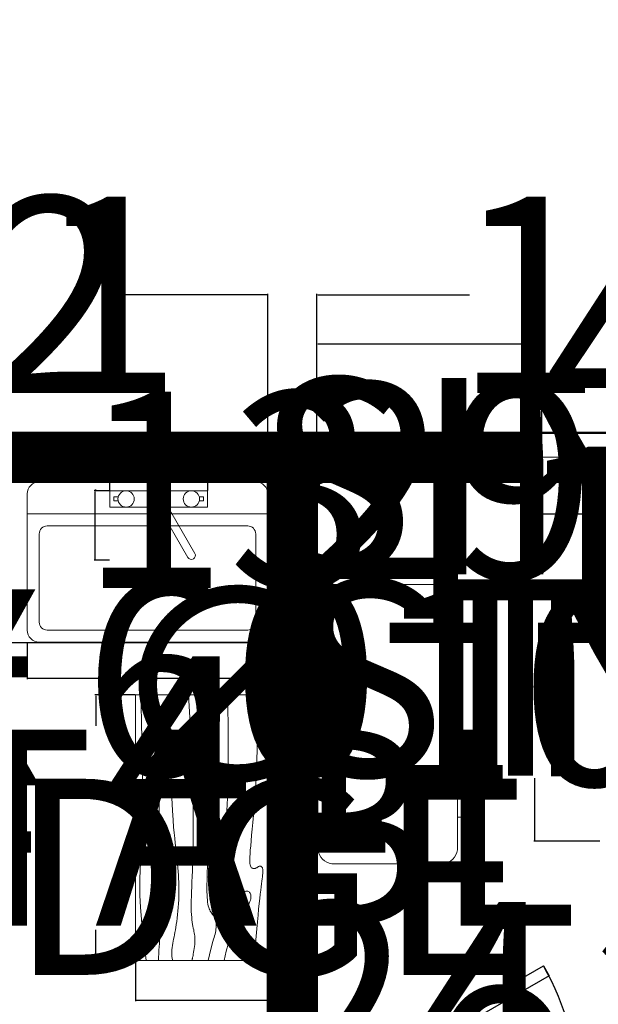
# Model space of a CAD drawing. Units: inches. Extents: x 1173 to 2157, y 515 to 1129.
# Tile 10 of 13: x 1475 to 1581, y 948 to 1129. Entities that reach past the tile are written whole.
import ezdxf

# ---------------------------------------------------------------- set-up
doc = ezdxf.new("R2010")
doc.units = ezdxf.units.IN
doc.header["$MEASUREMENT"] = 0
for name, color, linetype, lineweight in [('A-ANNO-DIMS', 2, 'Continuous', 18), ('A-DOOR', 3, 'Continuous', 25), ('A-FLOR-CASE', 32, 'Continuous', 25), ('A-FLOR-FIXT', 9, 'Continuous', 18), ('A-FURN', 8, 'Continuous', 18), ('A-GLAZ', 4, 'Continuous', 18), ('A-WALL', 7, 'Continuous', 50)]:
    doc.layers.add(name, color=color, linetype=linetype, lineweight=lineweight)
doc.layers.add('A-WALL-PATT', color=22, linetype='Continuous', lineweight=13, true_color=0xca4b0c)
doc.styles.get("Standard").update_dxf_attribs({"font": 'arial.ttf'})
doc.dimstyles.get("Standard").update_dxf_attribs({"dimtxt": 36, "dimasz": 0.18, "dimexe": 0.18, "dimexo": 0.0625, "dimgap": 0.09, "dimtad": 0, "dimtih": 1, "dimtoh": 1, "dimdec": 0, "dimrnd": 72, "dimzin": 0, "dimdsep": 46, "dimlunit": 3, "dimtxsty": 'Standard', "dimcen": 2, "dimadec": 0, "dimazin": 0, "dimtfac": 1, "dimtdec": 0, "dimtofl": 0, "dimtmove": 0, "dimatfit": 3, "dimfxl": 1, "dimtolj": 1, "dimtzin": 0, "dimarcsym": 0})

# ---------------------------------------------------------------- blocks, each defined once
blk = doc.blocks.new('*U3')
for p, q in [((0, 0), (0, -6)), ((40, 0), (40, -6))]:
    blk.add_line(p, q)
blk.add_lwpolyline([(0, 0), (34.64, 20), (35.52, 18.48), (0.88, -1.52)], close=True)
blk.add_arc((0, 0), 40, 0, 30)
blk = doc.blocks.new('Desk - 30 x 60 in.')
for p, q in [((-26.999995, 0), (26.999995, 0)), ((-29.999995, -27), (-29.999995, -3)), ((29.999995, -3), (29.999995, -27)), ((26.999995, -30), (-26.999995, -30)), ((-20.000005, -30), (-20.000005, -31)), ((-20.000005, -31), (-16.000005, -31)), ((-16.000005, -31), (-16.000005, -30)), ((15.999995, -31), (15.999995, -30)), ((19.999995, -31), (15.999995, -31)), ((19.999995, -30), (19.999995, -31))]:
    blk.add_line(p, q)
for centre, start, end in [((-26.499995, -3.5), 98.1301, 171.8699), ((26.499995, -3.5), 8.130102, 81.8699), ((-26.499995, -26.5), 188.1301, 261.8699), ((26.499995, -26.5), 278.1301, 351.8699)]:
    blk.add_arc(centre, 3.535534, start, end)
blk = doc.blocks.new('Table - Rectangular Woodgrain 60 x 30 in.')
for p, q in [((0, 0), (0, -30)), ((60, 0), (0, 0)), ((60, -30), (60, 0)), ((0, -30), (60, -30))]:
    blk.add_line(p, q)
for points in [[(0, -2.4), (4.8155, -2.418), (9.0302, -2.4688), (12.709, -2.5477), (15.9167, -2.65), (18.7181, -2.7711), (21.1781, -2.9063), (23.3616, -3.0508), (25.3333, -3.2), (27.1477, -3.3495), (28.8172, -3.4958), (30.3437, -3.636), (31.7291, -3.7667), (32.9756, -3.8849), (34.0849, -3.9875), (35.059, -4.0714), (35.9, -4.1334), (36.6114, -4.1711), (37.2041, -4.1854), (37.6906, -4.1779), (38.0833, -4.15), (38.3948, -4.1034), (38.6375, -4.0396), (38.8239, -3.9602), (38.9666, -3.8667), (39.0764, -3.7608), (39.1573, -3.6448), (39.2116, -3.521), (39.2416, -3.3917), (39.2498, -3.2593), (39.2385, -3.1261), (39.21, -2.9944), (39.1666, -2.8667), (39.111, -2.7447), (39.0468, -2.6281), (38.978, -2.5163), (38.9083, -2.4083), (38.8418, -2.3035), (38.7823, -2.201), (38.7337, -2.1001), (38.7, -2), (38.6844, -1.9003), (38.6875, -1.8021), (38.7094, -1.707), (38.75, -1.6167), (38.8094, -1.5326), (38.8875, -1.4563), (38.9844, -1.3893), (39.1, -1.3333), (39.2351, -1.2896), (39.3937, -1.2583), (39.5804, -1.2396), (39.8, -1.2333), (40.057, -1.2396), (40.3562, -1.2583), (40.7023, -1.2896), (41.1, -1.3333), (41.5547, -1.3895), (42.0755, -1.4573), (42.6721, -1.5361), (43.3542, -1.625), (44.1316, -1.7233), (45.014, -1.8302), (46.0114, -1.9449), (47.1333, -2.0667), (48.3862, -2.1947), (49.7625, -2.3281), (51.2513, -2.4663), (52.8416, -2.6083), (54.5226, -2.7535), (56.2833, -2.9011), (58.1127, -3.0501), (60, -3.2)], [(0, -9.2), (6.5759, -9.0858), (11.9385, -9.0365), (16.2527, -9.0418), (19.6833, -9.0917), (22.3952, -9.1759), (24.5531, -9.2844), (26.322, -9.4069), (27.8666, -9.5333), (29.3241, -9.6553), (30.7203, -9.7719), (32.0532, -9.8837), (33.3208, -9.9917), (34.5213, -10.0965), (35.6526, -10.199), (36.7128, -10.2999), (37.7, -10.4), (38.6129, -10.4996), (39.4531, -10.5969), (40.223, -10.6895), (40.925, -10.775), (41.5613, -10.8512), (42.1344, -10.9156), (42.6465, -10.966), (43.1, -11), (43.4976, -11.0158), (43.8437, -11.0136), (44.143, -10.9942), (44.4, -10.9583), (44.6195, -10.9069), (44.8062, -10.8406), (44.9648, -10.7603), (45.1, -10.6667), (45.2155, -10.5598), (45.3114, -10.4365), (45.3871, -10.2929), (45.4416, -10.125), (45.4743, -9.929), (45.4844, -9.7011), (45.4709, -9.4371), (45.4333, -9.1333), (45.3716, -8.7883), (45.2896, -8.4104), (45.1919, -8.0107), (45.0833, -7.6), (44.9685, -7.1893), (44.8521, -6.7896), (44.7388, -6.4117), (44.6333, -6.0667), (44.54, -5.7628), (44.4614, -5.4979), (44.4001, -5.2675), (44.3583, -5.0667), (44.3384, -4.8909), (44.3427, -4.7354), (44.3736, -4.5956), (44.4333, -4.4667), (44.5236, -4.3453), (44.6427, -4.2333), (44.7884, -4.1339), (44.9583, -4.05), (45.1501, -3.9849), (45.3614, -3.9417), (45.59, -3.9234), (45.8333, -3.9333), (46.0915, -3.9749), (46.3734, -4.0531), (46.6906, -4.1736), (47.0542, -4.3417), (47.4756, -4.5629), (47.9661, -4.8427), (48.5372, -5.1866), (49.2, -5.6), (49.9676, -6.0844), (50.8594, -6.625), (51.8965, -7.2031), (53.1, -7.8), (54.491, -8.3969), (56.0906, -8.975), (57.9199, -9.5156), (60, -10)], [(0, -12.8), (5.1847, -12.9322), (9.6213, -13.0323), (13.3963, -13.1059), (16.5958, -13.1583), (19.3063, -13.1952), (21.614, -13.2219), (23.6054, -13.2439), (25.3666, -13.2667), (26.9728, -13.2947), (28.4531, -13.3281), (29.8256, -13.3663), (31.1083, -13.4083), (32.3191, -13.4535), (33.476, -13.501), (34.597, -13.5501), (35.7, -13.6), (36.7984, -13.6497), (37.8875, -13.6979), (38.9578, -13.743), (40, -13.7833), (41.0047, -13.8174), (41.9625, -13.8438), (42.864, -13.8607), (43.7, -13.8667), (44.4631, -13.8604), (45.1552, -13.8417), (45.7801, -13.8104), (46.3416, -13.7667), (46.8439, -13.7104), (47.2906, -13.6417), (47.6858, -13.5604), (48.0333, -13.4667), (48.3375, -13.3608), (48.6042, -13.2448), (48.8396, -13.121), (49.05, -12.9917), (49.2417, -12.8593), (49.4208, -12.7261), (49.5937, -12.5944), (49.7667, -12.4667), (49.9452, -12.3451), (50.1323, -12.2313), (50.3303, -12.1268), (50.5416, -12.0333), (50.7686, -11.9524), (51.0135, -11.8854), (51.2788, -11.8341), (51.5666, -11.8), (51.8785, -11.7843), (52.2116, -11.7865), (52.562, -11.8059), (52.926, -11.8417), (53.2998, -11.8931), (53.6795, -11.9594), (54.0614, -12.0397), (54.4416, -12.1333), (54.8223, -12.2401), (55.2293, -12.3625), (55.6942, -12.5037), (56.2489, -12.6667), (56.9251, -12.8547), (57.7545, -13.0708), (58.7689, -13.3182), (60, -13.6)], [(0, -18), (5.124, -17.7273), (9.6609, -17.5057), (13.6705, -17.3303), (17.2125, -17.1958), (20.3467, -17.0973), (23.1328, -17.0297), (25.6307, -16.9878), (27.9, -16.9667), (29.9928, -16.9617), (31.9302, -16.9703), (33.7254, -16.9907), (35.3917, -17.0208), (36.9423, -17.0588), (38.3906, -17.1026), (39.7499, -17.1503), (41.0333, -17.2), (42.2519, -17.2496), (43.4073, -17.2969), (44.4986, -17.3395), (45.525, -17.375), (46.4858, -17.4012), (47.3802, -17.4156), (48.2074, -17.416), (48.9667, -17.4), (49.6583, -17.3662), (50.2872, -17.3167), (50.8595, -17.2547), (51.3812, -17.1833), (51.8584, -17.1057), (52.2971, -17.025), (52.7034, -16.9443), (53.0833, -16.8667), (53.443, -16.7951), (53.789, -16.7313), (54.128, -16.6768), (54.4666, -16.6334), (54.8115, -16.6024), (55.1693, -16.5854), (55.5465, -16.5841), (55.95, -16.6), (56.3828, -16.6337), (56.8346, -16.6823), (57.2915, -16.7418), (57.7396, -16.8084), (58.165, -16.878), (58.5539, -16.9469), (58.8924, -17.0111), (59.1666, -17.0667), (59.3679, -17.1107), (59.5078, -17.1438), (59.6032, -17.1675), (59.6708, -17.1833), (59.7275, -17.193), (59.7901, -17.1979), (59.8753, -17.1998), (60, -17.2)], [(0, -22.4), (8.0098, -22.2501), (14.4094, -22.1011), (19.4168, -21.9535), (23.25, -21.8083), (26.1269, -21.6663), (28.2656, -21.5281), (29.884, -21.3947), (31.2, -21.2667), (32.3967, -21.1448), (33.5172, -21.0292), (34.5697, -20.9198), (35.5625, -20.8167), (36.5037, -20.7198), (37.4015, -20.6292), (38.2642, -20.5448), (39.1, -20.4667), (39.9164, -20.3951), (40.7187, -20.3313), (41.5117, -20.2768), (42.3, -20.2333), (43.0883, -20.2024), (43.8812, -20.1854), (44.6836, -20.1841), (45.5, -20.2), (46.3328, -20.234), (47.1747, -20.2844), (48.0163, -20.3488), (48.8479, -20.425), (49.66, -20.5106), (50.4429, -20.6031), (51.1872, -20.7004), (51.8833, -20.8), (52.5246, -20.8999), (53.1166, -20.9995), (53.6681, -21.0983), (54.1875, -21.1958), (54.6834, -21.2919), (55.1646, -21.3859), (55.6394, -21.4777), (56.1167, -21.5667), (56.6028, -21.6515), (57.0961, -21.7266), (57.5929, -21.7852), (58.0896, -21.8208), (58.5823, -21.8268), (59.0674, -21.7964), (59.5412, -21.723), (60, -21.6)], [(0, -25.2), (8.6355, -25.0504), (15.7026, -24.9031), (21.4049, -24.7606), (25.9458, -24.625), (29.529, -24.4988), (32.3578, -24.3844), (34.6359, -24.284), (36.5667, -24.2), (38.3213, -24.1341), (39.9417, -24.0854), (41.437, -24.0523), (42.8167, -24.0333), (44.0901, -24.0268), (45.2667, -24.0313), (46.3557, -24.0451), (47.3667, -24.0667), (48.309, -24.0947), (49.1928, -24.1287), (50.0284, -24.168), (50.826, -24.2125), (51.5959, -24.2617), (52.3483, -24.3151), (53.0935, -24.3725), (53.8417, -24.4334), (54.6009, -24.497), (55.3699, -24.561), (56.1454, -24.6226), (56.9239, -24.6792), (57.7021, -24.7279), (58.4764, -24.7662), (59.2435, -24.7911), (60, -24.8)], [(0, -28.8), (5.6867, -28.6681), (10.45, -28.5698), (14.407, -28.5012), (17.675, -28.4584), (20.3711, -28.4374), (22.6125, -28.4344), (24.5164, -28.4455), (26.2, -28.4667), (27.762, -28.4947), (29.2276, -28.5281), (30.6033, -28.5663), (31.8958, -28.6084), (33.1118, -28.6535), (34.2578, -28.7011), (35.3405, -28.7501), (36.3666, -28.8), (37.3443, -28.8497), (38.288, -28.8974), (39.2137, -28.9412), (40.1375, -28.9792), (41.0753, -29.0093), (42.0432, -29.0297), (43.0572, -29.0384), (44.1333, -29.0333), (45.2936, -29.0114), (46.5843, -28.9641), (48.0579, -28.8816), (49.7666, -28.7542), (51.7629, -28.5721), (54.0989, -28.3255), (56.8272, -28.0048), (60, -27.6)]]:
    blk.add_lwpolyline(points)
blk = doc.blocks.new('Sink-single - 30 in top')
blk.add_line((-15, -3.999996), (15, -3.999996))
for points in [[(-13.5, 0), (13.5, 0)], [(-15, -18.499996), (-15, -1.5)], [(15, -1.5), (15, -18.499996)], [(-12.5, -5.499996), (12.5, -5.499996)], [(-13.5, -17.499996), (-13.5, -6.499996)], [(13.5, -6.499996), (13.5, -17.499996)], [(12.5, -18.499996), (-12.5, -18.499996)], [(13.5, -19.999996), (-13.5, -19.999996)]]:
    blk.add_lwpolyline(points)
for radius in [1, 0.5]:
    blk.add_circle((0, -11.999996), radius)
for centre, radius, start, end in [((-13.5, -1.5), 1.5, 90, 180), ((13.5, -1.5), 1.5, 0, 90), ((-12.5, -6.499996), 1, 90, 180), ((12.5, -6.499996), 1, 0, 90), ((-12.5, -17.499996), 1, 180, 270), ((12.5, -17.499996), 1, 270, 0), ((-13.5, -18.499996), 1.5, 180, 270), ((13.5, -18.499996), 1.5, 270, 0)]:
    blk.add_arc(centre, radius, start, end)
blk = doc.blocks.new('Faucet - kit sink top')
for p, q in [((-5.5, -0.75), (-5.5, -1.25)), ((-4.94278, -0.75), (-5.5, -0.75)), ((4.94278, -0.75), (5.5, -0.75)), ((5.5, -0.75), (5.5, -1.25)), ((-5.5, -1.25), (-4.94278, -1.25)), ((-0.14775, -1.7441), (3.56698, -8.1782)), ((4.43301, -7.6782), (0.71828, -1.2441)), ((5.5, -1.25), (4.94278, -1.25))]:
    blk.add_line(p, q)
blk.add_lwpolyline([(-0.00587, -2), (-6, -2), (-6, 0), (6, 0), (6, -2), (1.15195, -2)])
for centre, radius in [((-4, -1), 1), ((4, -1), 1), ((0, -1), 0.75)]:
    blk.add_circle(centre, radius)
blk.add_arc((4, -7.9282), 0.5, 210, 30)
blk = doc.blocks.new('WIN-48X9')
blk.add_line((48, 4.5), (0, 4.5))
blk.add_lwpolyline([(0, 9), (48, 9), (48, 0), (0, 0)], close=True)
blk = doc.blocks.new('*D29')
at = {"layer": 'A-ANNO-DIMS', "color": 0, "lineweight": -2, "transparency": 16777216}
for p, q in [((1581.6, 1038.37), (1569.48, 1038.37)), ((1569.66, 1038.19), (1569.66, 1026.84)), ((1569.66, 978.55), (1569.66, 989.9)), ((1581.6, 978.37), (1569.48, 978.37))]:
    blk.add_line(p, q, dxfattribs=at)
at = {"layer": 'A-ANNO-DIMS', "color": 0, "transparency": 16777216}
for points in [[(1569.63, 1038.19), (1569.69, 1038.19), (1569.66, 1038.37)], [(1569.63, 978.55), (1569.69, 978.55), (1569.66, 978.37)]]:
    blk.add_solid(points, dxfattribs=at)
at = {"layer": 'Defpoints', "color": 0, "transparency": 16777216}
for p in [(1581.66, 1038.37), (1569.66, 978.37), (1581.66, 978.37)]:
    blk.add_point(p, dxfattribs=at)
at = {"layer": 'A-ANNO-DIMS', "color": 0, "transparency": 16777216, "insert": (1569.66, 1008.37), "char_height": 36, "attachment_point": 5}
blk.add_mtext('\\A1;60 TYP.', dxfattribs=at)
blk = doc.blocks.new('*D36')
at = {"layer": 'A-ANNO-DIMS', "color": 0, "lineweight": -2, "transparency": 16777216}
for p, q in [((1497.87, 905.02), (1487.37, 905.02)), ((1487.55, 904.84), (1487.55, 889.09)), ((1487.55, 835.93), (1487.55, 851.68)), ((1497.87, 835.75), (1487.37, 835.75))]:
    blk.add_line(p, q, dxfattribs=at)
at = {"layer": 'A-ANNO-DIMS', "color": 0, "transparency": 16777216}
for points in [[(1487.52, 904.84), (1487.58, 904.84), (1487.55, 905.02)], [(1487.52, 835.93), (1487.58, 835.93), (1487.55, 835.75)]]:
    blk.add_solid(points, dxfattribs=at)
at = {"layer": 'Defpoints', "color": 0, "transparency": 16777216}
for p in [(1497.94, 905.02), (1487.55, 835.75), (1497.94, 835.75)]:
    blk.add_point(p, dxfattribs=at)
at = {"layer": 'A-ANNO-DIMS', "color": 0, "transparency": 16777216, "insert": (1487.55, 870.38), "char_height": 36, "attachment_point": 5}
blk.add_mtext('\\A1;DINING SET 69', dxfattribs=at)
blk = doc.blocks.new('*D46')
at = {"layer": 'A-ANNO-DIMS', "color": 0, "lineweight": -2, "transparency": 16777216}
for p, q in [((1646.37, 911.98), (1645.86, 896.32)), ((1648.72, 912.09), (1646.2, 912.17)), ((1648.2, 896.07), (1645.68, 896.15)), ((1645.86, 896.14), (1645.85, 895.96)), ((1645.85, 895.96), (1645.67, 895.96))]:
    blk.add_line(p, q, dxfattribs=at)
at = {"layer": 'A-ANNO-DIMS', "color": 0, "transparency": 16777216}
for points in [[(1646.34, 911.99), (1646.4, 911.98), (1646.38, 912.16)], [(1645.83, 896.32), (1645.89, 896.32), (1645.86, 896.14)]]:
    blk.add_solid(points, dxfattribs=at)
at = {"layer": 'Defpoints', "color": 0, "transparency": 16777216}
for p in [(1648.78, 912.09), (1645.86, 896.14), (1648.26, 896.06)]:
    blk.add_point(p, dxfattribs=at)
at = {"layer": 'A-ANNO-DIMS', "color": 0, "transparency": 16777216, "insert": (1538.16, 895.96), "char_height": 36, "attachment_point": 5}
blk.add_mtext('\\A1;BASIN 16', dxfattribs=at)
blk = doc.blocks.new('*D54')
at = {"layer": 'A-ANNO-DIMS', "color": 0, "lineweight": -2, "transparency": 16777216}
for p, q in [((1496.35, 1005.18), (1488.93, 1005.18)), ((1489.11, 1005), (1489.11, 999.54)), ((1489.11, 956.65), (1489.11, 962.11)), ((1496.35, 956.47), (1488.93, 956.47))]:
    blk.add_line(p, q, dxfattribs=at)
at = {"layer": 'A-ANNO-DIMS', "color": 0, "transparency": 16777216}
for points in [[(1489.08, 1005), (1489.14, 1005), (1489.11, 1005.18)], [(1489.08, 956.65), (1489.14, 956.65), (1489.11, 956.47)]]:
    blk.add_solid(points, dxfattribs=at)
at = {"layer": 'Defpoints', "color": 0, "transparency": 16777216}
for p in [(1496.42, 1005.18), (1489.11, 956.47), (1496.42, 956.47)]:
    blk.add_point(p, dxfattribs=at)
at = {"layer": 'A-ANNO-DIMS', "color": 0, "transparency": 16777216, "insert": (1489.11, 980.83), "char_height": 36, "attachment_point": 5}
blk.add_mtext('\\A1;WORK TABLE 49', dxfattribs=at)
blk = doc.blocks.new('*D55')
at = {"layer": 'A-ANNO-DIMS', "color": 0, "lineweight": -2, "transparency": 16777216}
for p, q in [((1496.42, 956.41), (1496.42, 948.98)), ((1520.77, 956.41), (1520.77, 948.98)), ((1496.6, 949.16), (1520.59, 949.16)), ((1520.77, 949.16), (1520.95, 949.16))]:
    blk.add_line(p, q, dxfattribs=at)
at = {"layer": 'A-ANNO-DIMS', "color": 0, "transparency": 16777216}
for points in [[(1496.6, 949.19), (1496.6, 949.13), (1496.42, 949.16)], [(1520.59, 949.19), (1520.59, 949.13), (1520.77, 949.16)]]:
    blk.add_solid(points, dxfattribs=at)
at = {"layer": 'Defpoints', "color": 0, "transparency": 16777216}
for p in [(1496.42, 956.47), (1520.77, 956.47), (1520.77, 949.16)]:
    blk.add_point(p, dxfattribs=at)
at = {"layer": 'A-ANNO-DIMS', "color": 0, "transparency": 16777216, "insert": (1547.06, 949.16), "char_height": 36, "attachment_point": 5}
blk.add_mtext('\\A1;24', dxfattribs=at)
blk = doc.blocks.new('*D56')
at = {"layer": 'A-ANNO-DIMS', "color": 0, "lineweight": -2, "transparency": 16777216}
for p, q in [((1426.92, 1014.79), (1433.2, 1014.79)), ((1433.02, 1014.61), (1433.02, 1012.98)), ((1433.02, 973.94), (1433.02, 975.57)), ((1426.92, 973.76), (1433.2, 973.76))]:
    blk.add_line(p, q, dxfattribs=at)
at = {"layer": 'A-ANNO-DIMS', "color": 0, "transparency": 16777216}
for points in [[(1432.99, 1014.61), (1433.05, 1014.61), (1433.02, 1014.79)], [(1432.99, 973.94), (1433.05, 973.94), (1433.02, 973.76)]]:
    blk.add_solid(points, dxfattribs=at)
at = {"layer": 'Defpoints', "color": 0, "transparency": 16777216}
for p in [(1426.86, 1014.79), (1433.02, 1014.79), (1426.86, 973.76)]:
    blk.add_point(p, dxfattribs=at)
at = {"layer": 'A-ANNO-DIMS', "color": 0, "transparency": 16777216, "insert": (1433.02, 994.27), "char_height": 36, "attachment_point": 5}
blk.add_mtext('\\A1;RANGE 41', dxfattribs=at)
blk = doc.blocks.new('*D58')
at = {"layer": 'A-ANNO-DIMS', "color": 0, "lineweight": -2, "transparency": 16777216}
for p, q in [((1476.55, 1014.81), (1476.55, 1008.07)), ((1520.66, 1014.81), (1520.66, 1008.07)), ((1476.73, 1008.25), (1520.48, 1008.25)), ((1520.66, 1008.25), (1520.84, 1008.25))]:
    blk.add_line(p, q, dxfattribs=at)
at = {"layer": 'A-ANNO-DIMS', "color": 0, "transparency": 16777216}
for points in [[(1476.73, 1008.28), (1476.73, 1008.22), (1476.55, 1008.25)], [(1520.48, 1008.28), (1520.48, 1008.22), (1520.66, 1008.25)]]:
    blk.add_solid(points, dxfattribs=at)
at = {"layer": 'Defpoints', "color": 0, "transparency": 16777216}
for p in [(1476.55, 1014.87), (1520.66, 1014.87), (1520.66, 1008.25)]:
    blk.add_point(p, dxfattribs=at)
at = {"layer": 'A-ANNO-DIMS', "color": 0, "transparency": 16777216, "insert": (1612.23, 1008.25), "char_height": 36, "attachment_point": 5}
blk.add_mtext('\\A1;SINK 44', dxfattribs=at)
blk = doc.blocks.new('*D59')
at = {"layer": 'A-ANNO-DIMS', "color": 0, "lineweight": -2, "transparency": 16777216}
for p, q in [((1520.73, 1044.28), (1527.46, 1044.28)), ((1527.28, 1044.28), (1527.28, 1044.46)), ((1527.28, 1044.46), (1527.46, 1044.46)), ((1527.28, 1015.05), (1527.28, 1044.1)), ((1520.73, 1014.87), (1527.46, 1014.87))]:
    blk.add_line(p, q, dxfattribs=at)
at = {"layer": 'A-ANNO-DIMS', "color": 0, "transparency": 16777216}
for points in [[(1527.25, 1044.1), (1527.31, 1044.1), (1527.28, 1044.28)], [(1527.25, 1015.05), (1527.31, 1015.05), (1527.28, 1014.87)]]:
    blk.add_solid(points, dxfattribs=at)
at = {"layer": 'Defpoints', "color": 0, "transparency": 16777216}
for p in [(1520.66, 1044.28), (1527.28, 1044.28), (1520.66, 1014.87)]:
    blk.add_point(p, dxfattribs=at)
at = {"layer": 'A-ANNO-DIMS', "color": 0, "transparency": 16777216, "insert": (1553.68, 1044.46), "char_height": 36, "attachment_point": 5}
blk.add_mtext('\\A1;29', dxfattribs=at)
blk = doc.blocks.new('*D60')
at = {"layer": 'A-ANNO-DIMS', "color": 0, "lineweight": -2, "transparency": 16777216}
for p, q in [((1396.06, 971.62), (1390.55, 971.62)), ((1390.73, 971.62), (1390.73, 971.8)), ((1390.73, 971.8), (1390.91, 971.8)), ((1390.73, 935.8), (1390.73, 971.44)), ((1396.06, 935.62), (1390.55, 935.62))]:
    blk.add_line(p, q, dxfattribs=at)
at = {"layer": 'A-ANNO-DIMS', "color": 0, "transparency": 16777216}
for points in [[(1390.7, 971.44), (1390.76, 971.44), (1390.73, 971.62)], [(1390.7, 935.8), (1390.76, 935.8), (1390.73, 935.62)]]:
    blk.add_solid(points, dxfattribs=at)
at = {"layer": 'Defpoints', "color": 0, "transparency": 16777216}
for p in [(1390.73, 971.62), (1396.13, 971.62), (1396.13, 935.62)]:
    blk.add_point(p, dxfattribs=at)
at = {"layer": 'A-ANNO-DIMS', "color": 0, "transparency": 16777216, "insert": (1517.73, 971.8), "char_height": 36, "attachment_point": 5}
blk.add_mtext('\\A1;FRIDGE 36', dxfattribs=at)
blk = doc.blocks.new('*D62')
at = {"layer": 'A-ANNO-DIMS', "color": 0, "lineweight": -2, "transparency": 16777216}
for p, q in [((1491.7, 1042.71), (1491.7, 1045.52)), ((1491.88, 1045.34), (1509.47, 1045.34)), ((1509.65, 1042.71), (1509.65, 1045.52)), ((1509.65, 1045.34), (1509.83, 1045.34))]:
    blk.add_line(p, q, dxfattribs=at)
at = {"layer": 'A-ANNO-DIMS', "color": 0, "transparency": 16777216}
for points in [[(1491.88, 1045.37), (1491.88, 1045.31), (1491.7, 1045.34)], [(1509.47, 1045.37), (1509.47, 1045.31), (1509.65, 1045.34)]]:
    blk.add_solid(points, dxfattribs=at)
at = {"layer": 'Defpoints', "color": 0, "transparency": 16777216}
for p in [(1509.65, 1045.34), (1491.7, 1042.65), (1509.65, 1042.65)]:
    blk.add_point(p, dxfattribs=at)
at = {"layer": 'A-ANNO-DIMS', "color": 0, "transparency": 16777216, "insert": (1657.22, 1045.34), "char_height": 36, "attachment_point": 5}
blk.add_mtext('\\A1;SINK TAP 18', dxfattribs=at)
blk = doc.blocks.new('*D63')
at = {"layer": 'A-ANNO-DIMS', "color": 0, "lineweight": -2, "transparency": 16777216}
for p, q in [((1491.63, 1042.65), (1488.82, 1042.65)), ((1489, 1042.65), (1489, 1042.83)), ((1489, 1042.83), (1489.18, 1042.83)), ((1489, 1030.11), (1489, 1042.47)), ((1491.63, 1029.93), (1488.82, 1029.93))]:
    blk.add_line(p, q, dxfattribs=at)
at = {"layer": 'A-ANNO-DIMS', "color": 0, "transparency": 16777216}
for points in [[(1488.97, 1042.47), (1489.03, 1042.47), (1489, 1042.65)], [(1488.97, 1030.11), (1489.03, 1030.11), (1489, 1029.93)]]:
    blk.add_solid(points, dxfattribs=at)
at = {"layer": 'Defpoints', "color": 0, "transparency": 16777216}
for p in [(1489, 1042.65), (1491.7, 1042.65), (1491.7, 1029.93)]:
    blk.add_point(p, dxfattribs=at)
at = {"layer": 'A-ANNO-DIMS', "color": 0, "transparency": 16777216, "insert": (1513.36, 1042.83), "char_height": 36, "attachment_point": 5}
blk.add_mtext('\\A1;13', dxfattribs=at)
blk = doc.blocks.new('*D67')
at = {"layer": 'A-ANNO-DIMS', "color": 0, "lineweight": -2, "transparency": 16777216}
for p, q in [((1388.66, 1044.34), (1388.66, 1078.79)), ((1388.84, 1078.61), (1416.68, 1078.61)), ((1520.48, 1078.61), (1492.64, 1078.61)), ((1520.66, 1044.34), (1520.66, 1078.79))]:
    blk.add_line(p, q, dxfattribs=at)
at = {"layer": 'A-ANNO-DIMS', "color": 0, "transparency": 16777216}
for points in [[(1388.84, 1078.64), (1388.84, 1078.58), (1388.66, 1078.61)], [(1520.48, 1078.64), (1520.48, 1078.58), (1520.66, 1078.61)]]:
    blk.add_solid(points, dxfattribs=at)
at = {"layer": 'Defpoints', "color": 0, "transparency": 16777216}
for p in [(1520.66, 1078.61), (1388.66, 1044.28), (1520.66, 1044.28)]:
    blk.add_point(p, dxfattribs=at)
at = {"layer": 'A-ANNO-DIMS', "color": 0, "transparency": 16777216, "insert": (1454.66, 1078.61), "char_height": 36, "attachment_point": 5}
blk.add_mtext('\\A1;132', dxfattribs=at)
blk = doc.blocks.new('*D68')
at = {"layer": 'A-ANNO-DIMS', "color": 0, "lineweight": -2, "transparency": 16777216}
for p, q in [((1379.66, 1053.34), (1379.66, 1078.79)), ((1379.84, 1078.61), (1413.58, 1078.61)), ((1413.76, 1053.34), (1413.76, 1078.79)), ((1413.76, 1078.61), (1413.94, 1078.61))]:
    blk.add_line(p, q, dxfattribs=at)
at = {"layer": 'A-ANNO-DIMS', "color": 0, "transparency": 16777216}
for points in [[(1379.84, 1078.64), (1379.84, 1078.58), (1379.66, 1078.61)], [(1413.58, 1078.64), (1413.58, 1078.58), (1413.76, 1078.61)]]:
    blk.add_solid(points, dxfattribs=at)
at = {"layer": 'Defpoints', "color": 0, "transparency": 16777216}
for p in [(1413.76, 1078.61), (1379.66, 1053.28), (1413.76, 1053.28)]:
    blk.add_point(p, dxfattribs=at)
at = {"layer": 'A-ANNO-DIMS', "color": 0, "transparency": 16777216, "insert": (1457.3, 1078.61), "char_height": 36, "attachment_point": 5}
blk.add_mtext('\\A1;34.1', dxfattribs=at)
blk = doc.blocks.new('*D88')
at = {"layer": 'A-ANNO-DIMS', "color": 0, "lineweight": -2, "transparency": 16777216}
for p, q in [((1529.66, 1044.34), (1529.65, 1069.76)), ((1529.83, 1069.58), (1570.76, 1069.61)), ((1570.95, 1044.37), (1570.94, 1069.79)), ((1570.94, 1069.61), (1571.12, 1069.61))]:
    blk.add_line(p, q, dxfattribs=at)
at = {"layer": 'A-ANNO-DIMS', "color": 0, "transparency": 16777216}
for points in [[(1529.83, 1069.61), (1529.83, 1069.55), (1529.65, 1069.58)], [(1570.76, 1069.64), (1570.76, 1069.58), (1570.94, 1069.61)]]:
    blk.add_solid(points, dxfattribs=at)
at = {"layer": 'Defpoints', "color": 0, "transparency": 16777216}
for p in [(1570.94, 1069.61), (1529.66, 1044.28), (1570.95, 1044.31)]:
    blk.add_point(p, dxfattribs=at)
at = {"layer": 'A-ANNO-DIMS', "color": 0, "transparency": 16777216, "insert": (1632.71, 1069.61), "char_height": 36, "attachment_point": 5}
blk.add_mtext('\\A1;41.29', dxfattribs=at)
blk = doc.blocks.new('*D89')
at = {"layer": 'A-ANNO-DIMS', "color": 0, "lineweight": -2, "transparency": 16777216}
for p, q in [((1529.66, 1044.34), (1529.66, 1078.79)), ((1529.84, 1078.61), (1557.68, 1078.61)), ((1661.48, 1078.61), (1633.64, 1078.61)), ((1661.66, 1044.34), (1661.66, 1078.79))]:
    blk.add_line(p, q, dxfattribs=at)
at = {"layer": 'A-ANNO-DIMS', "color": 0, "transparency": 16777216}
for points in [[(1529.84, 1078.64), (1529.84, 1078.58), (1529.66, 1078.61)], [(1661.48, 1078.64), (1661.48, 1078.58), (1661.66, 1078.61)]]:
    blk.add_solid(points, dxfattribs=at)
at = {"layer": 'Defpoints', "color": 0, "transparency": 16777216}
for p in [(1661.66, 1078.61), (1529.66, 1044.28), (1661.66, 1044.28)]:
    blk.add_point(p, dxfattribs=at)
at = {"layer": 'A-ANNO-DIMS', "color": 0, "transparency": 16777216, "insert": (1595.66, 1078.61), "char_height": 36, "attachment_point": 5}
blk.add_mtext('\\A1;132', dxfattribs=at)
blk = doc.blocks.new('*D91')
at = {"layer": 'A-ANNO-DIMS', "color": 0, "lineweight": -2, "transparency": 16777216}
for p, q in [((1661.73, 1044.28), (1687.15, 1044.28)), ((1686.97, 1044.1), (1686.97, 1033.07)), ((1661.73, 1032.89), (1687.15, 1032.89)), ((1686.97, 1032.71), (1686.79, 1032.71)), ((1686.97, 1032.89), (1686.97, 1032.71))]:
    blk.add_line(p, q, dxfattribs=at)
at = {"layer": 'A-ANNO-DIMS', "color": 0, "transparency": 16777216}
for points in [[(1686.94, 1044.1), (1687, 1044.1), (1686.97, 1044.28)], [(1686.94, 1033.07), (1687, 1033.07), (1686.97, 1032.89)]]:
    blk.add_solid(points, dxfattribs=at)
at = {"layer": 'Defpoints', "color": 0, "transparency": 16777216}
for p in [(1661.66, 1044.28), (1661.66, 1032.89), (1686.97, 1032.89)]:
    blk.add_point(p, dxfattribs=at)
at = {"layer": 'A-ANNO-DIMS', "color": 0, "transparency": 16777216, "insert": (1613.66, 1032.71), "char_height": 36, "attachment_point": 5}
blk.add_mtext('\\A1;11.393', dxfattribs=at)
blk = doc.blocks.new('*D94')
at = {"layer": 'A-ANNO-DIMS', "color": 0, "lineweight": -2, "transparency": 16777216}
for p, q in [((1577.6, 933.28), (1552.18, 933.28)), ((1552.36, 933.28), (1552.36, 933.46)), ((1552.36, 933.46), (1552.54, 933.46)), ((1552.36, 924.46), (1552.36, 933.1)), ((1577.6, 924.28), (1552.18, 924.28))]:
    blk.add_line(p, q, dxfattribs=at)
at = {"layer": 'A-ANNO-DIMS', "color": 0, "transparency": 16777216}
for points in [[(1552.33, 933.1), (1552.39, 933.1), (1552.36, 933.28)], [(1552.33, 924.46), (1552.39, 924.46), (1552.36, 924.28)]]:
    blk.add_solid(points, dxfattribs=at)
at = {"layer": 'Defpoints', "color": 0, "transparency": 16777216}
for p in [(1552.36, 933.28), (1577.66, 933.28), (1577.66, 924.28)]:
    blk.add_point(p, dxfattribs=at)
at = {"layer": 'A-ANNO-DIMS', "color": 0, "transparency": 16777216, "insert": (1564.47, 933.46), "char_height": 36, "attachment_point": 5}
blk.add_mtext('\\A1;9', dxfattribs=at)
blk = doc.blocks.new('*D107')
at = {"layer": 'A-ANNO-DIMS', "color": 0, "lineweight": -2, "transparency": 16777216}
for p, q in [((1607.48, 928.68), (1607.66, 928.68)), ((1607.66, 928.68), (1607.66, 920.46)), ((1607.66, 904.28), (1607.66, 908.28)), ((1605.66, 906.28), (1609.66, 906.28))]:
    blk.add_line(p, q, dxfattribs=at)
at = {"layer": 'A-ANNO-DIMS', "color": 0, "transparency": 16777216}
blk.add_solid([(1607.69, 920.46), (1607.63, 920.46), (1607.66, 920.28)], dxfattribs=at)
at = {"layer": 'Defpoints', "color": 0, "transparency": 16777216}
for p in [(1607.66, 920.28), (1607.66, 906.28)]:
    blk.add_point(p, dxfattribs=at)
at = {"layer": 'A-ANNO-DIMS', "color": 0, "transparency": 16777216, "insert": (1564.46, 928.68), "char_height": 36, "attachment_point": 5}
blk.add_mtext('\\A1;R14', dxfattribs=at)
blk = doc.blocks.new('*D110')
at = {"layer": 'A-ANNO-DIMS', "color": 0, "lineweight": -2, "transparency": 16777216}
for p, q in [((1415.92, 1004.58), (1415.92, 1008.58)), ((1413.92, 1006.58), (1417.92, 1006.58)), ((1424.67, 1006.58), (1421.57, 1006.58))]:
    blk.add_line(p, q, dxfattribs=at)
at = {"layer": 'A-ANNO-DIMS', "color": 0, "transparency": 16777216}
blk.add_solid([(1421.57, 1006.61), (1421.57, 1006.55), (1421.39, 1006.58)], dxfattribs=at)
at = {"layer": 'Defpoints', "color": 0, "transparency": 16777216}
for p in [(1410.45, 1006.58), (1421.39, 1006.58)]:
    blk.add_point(p, dxfattribs=at)
at = {"layer": 'A-ANNO-DIMS', "color": 0, "transparency": 16777216, "insert": (1556.91, 1006.58), "char_height": 36, "attachment_point": 5}
blk.add_mtext('\\A1;2X ∅10.942', dxfattribs=at)

msp = doc.modelspace()

# ---------------------------------------------------------------- hatches: boundary and pattern name
at = {"layer": 'A-WALL-PATT'}
h = msp.add_hatch(dxfattribs=at)
h.set_pattern_fill('ANSI31', color=256)
h.paths.add_polyline_path([(1388.6635, 933.2805), (1388.6635, 1044.2805), (1413.7618, 1044.2805), (1413.7618, 1053.2805), (1379.6635, 1053.2805), (1379.6635, 894.1606), (1388.6635, 894.1606), (1388.6635, 924.2805), (1472.6635, 924.2805), (1472.6635, 933.2805)])
h.paths.add_polyline_path([(1520.6635, 1044.2805), (1520.6635, 1014.7866), (1520.6635, 1005.1794), (1520.7714, 1005.1794), (1520.7714, 956.4707), (1520.6635, 924.2805), (1529.6635, 924.2805), (1529.6635, 931.4788), (1529.6635, 1044.2805), (1530.8474, 1044.2805), (1570.9543, 1044.2805), (1570.9543, 1053.2805), (1461.7618, 1053.2805), (1461.7618, 1044.2805)])
h.paths.add_polyline_path([(1618.9543, 1053.2805), (1618.9543, 1044.2805), (1661.6635, 1044.2805), (1661.6635, 1043.7367), (1661.6635, 1032.8874), (1670.6635, 1032.8874), (1670.6635, 1053.2805)])
h.paths.add_polyline_path([(1661.6635, 933.2805), (1661.6635, 927.8377), (1661.6635, 924.2805), (1661.6635, 918.9156), (1670.6635, 918.9156), (1670.6635, 984.8874), (1661.6635, 984.8874), (1661.6635, 978.3712)])
h.paths.add_polyline_path([(1670.6635, 894.9156), (1661.6635, 894.9156), (1661.6635, 890.0349), (1661.9328, 890.0349), (1661.9328, 870.079), (1661.6635, 864.2805), (1589.6635, 864.2805), (1589.6635, 924.2805), (1625.553, 924.2805, -0.02455299), (1625.3782, 927.8377), (1625.3782, 933.2805), (1577.6635, 933.2805), (1577.6635, 924.2805), (1580.6635, 924.2805), (1580.6635, 855.2805), (1586.1062, 855.2805), (1589.6635, 855.2805), (1661.6635, 855.2805), (1661.6635, 826.5597), (1670.6635, 826.5597)])
h.paths.add_polyline_path([(1670.6635, 802.5597), (1661.6635, 802.5597), (1661.6635, 795.2805), (1589.6635, 795.2805), (1589.6635, 819.17, -0.02455299), (1586.1062, 818.9952), (1580.6635, 818.9952), (1580.6635, 795.2805), (1577.6635, 795.2805), (1577.6635, 786.2805), (1661.6635, 786.2805), (1661.6635, 778.5597), (1661.6635, 742.6973), (1670.6635, 742.6973)])
h.paths.add_polyline_path([(1661.6635, 654.2805), (1625.1498, 654.2805), (1625.1498, 645.2805), (1661.3656, 645.2805), (1661.6635, 645.2805), (1661.6635, 573.2805), (1520.6635, 573.2805), (1520.6635, 564.2805), (1670.6635, 564.2805), (1670.6635, 694.6973), (1661.6635, 694.6973)])
h.paths.add_polyline_path([(1529.4367, 733.4702, -0.06854064), (1529.6635, 734.2623), (1529.6635, 795.2805), (1520.6635, 795.2805), (1520.6635, 645.2805), (1577.1498, 645.2805), (1577.1498, 654.2805), (1529.6635, 654.2805), (1529.6635, 686.5626, -0.06854064), (1529.4367, 687.3547)])
h.paths.add_polyline_path([(1379.6635, 711.2805), (1388.6635, 711.2805), (1458.7214, 711.2805), (1458.7214, 720.2805), (1410.7214, 720.2805), (1388.6635, 720.2805), (1388.6635, 745.0427), (1379.6635, 745.0427)])
h.paths.add_polyline_path([(1388.6635, 846.1606), (1379.6635, 846.1606), (1379.6635, 793.0427), (1388.6635, 793.0427)])

# ---------------------------------------------------------------- linework, layer by layer
at = {"layer": 'A-FLOR-CASE'}
msp.add_lwpolyline([(1424.1251, 1014.7866), (1520.6635, 1014.7866), (1520.6635, 1044.2805), (1388.6635, 1044.2805), (1388.6635, 1014.7866)], dxfattribs=at)
at = {"layer": 'A-WALL'}
for p, q in [((1520.6635, 1044.2805), (1388.6635, 1044.2805)), ((1520.0174, 1044.2805), (1520.6635, 1044.2805)), ((1520.6635, 924.2805), (1520.6635, 1044.2805)), ((1661.6635, 1044.2805), (1529.6635, 1044.2805)), ((1529.6635, 924.2805), (1529.6635, 1044.2805)), ((1529.6635, 924.2805), (1529.6635, 1044.2805)), ((1529.6635, 1044.2805), (1530.8474, 1044.2805))]:
    msp.add_line(p, q, dxfattribs=at)
msp.add_lwpolyline([(1379.6635, 564.2805), (1670.6635, 564.2805), (1670.6635, 1053.2805), (1379.6635, 1053.2805)], close=True, dxfattribs=at)

# ---------------------------------------------------------------- block references
at = {"layer": 'A-DOOR', "xscale": 1.199708577982686, "yscale": 1.199708577982686, "zscale": 1.199708577982686}
msp.add_blockref('*U3', (1529.6635, 931.4788), dxfattribs=at)
at = {"layer": 'A-FLOR-FIXT'}
for name, p, xscale, yscale, zscale in [('Sink-single - 30 in top', (1498.605, 1044.2805), 1.470565744207578, 1.470565744207578, 1.470565744207578), ('Faucet - kit sink top', (1500.6707, 1042.6479), 1.495937695643116, 1.495937695643116, 1.495937695643116)]:
    msp.add_blockref(name, p, dxfattribs=dict(at, xscale=xscale, yscale=yscale, zscale=zscale))
at = {"layer": 'A-FURN'}
for name, p, xscale, yscale, zscale, rotation in [('Desk - 30 x 60 in.', (1529.8706, 999.8191), 0.8539907571596934, 0.8539907571596934, 0.8539907571596934, 90), ('Table - Rectangular Woodgrain 60 x 30 in.', (1520.7714, 1005.1794), 0.8118122773479608, 0.8118122773479608, 0.8118122773479608, 270)]:
    msp.add_blockref(name, p, dxfattribs=dict(at, xscale=xscale, yscale=yscale, zscale=zscale, rotation=rotation))
at = {"layer": 'A-GLAZ'}
msp.add_blockref('WIN-48X9', (1570.9543, 1044.3102), dxfattribs=at)

# ---------------------------------------------------------------- dimensions: what is measured, and where the dimension line sits
at = {"layer": 'A-ANNO-DIMS'}
for base, p1, p2, text, picture, middle in [((1509.6463, 1045.3406), (1491.6951, 1042.6479), (1509.6463, 1042.6479), 'SINK TAP <>', '*D62', (1657.2192, 1045.3406)), ((1520.6635, 1008.2517), (1476.5465, 1014.8692), (1520.6635, 1014.8692), 'SINK <>', '*D58', (1612.235, 1008.2517))]:
    dim = msp.add_linear_dim(base=base, p1=p1, p2=p2, text=text, dimstyle='Standard', override={"dimdec": 0, "dimlfac": 1, "dimrnd": 0, "dimzin": 0, "dimdsep": 46, "dimlunit": 2}, dxfattribs=at)
    dim.commit()
    dim.dimension.update_dxf_attribs({"geometry": picture, "text_midpoint": middle})
for base, p1, p2, override, picture, middle in [((1413.7618, 1078.6127), (1379.6635, 1053.2805), (1413.7618, 1053.2805), {"dimdec": 1, "dimlfac": 1, "dimrnd": 0, "dimzin": 0, "dimdsep": 46, "dimlunit": 2}, '*D68', (1457.3006, 1078.6127)), ((1520.6635, 1078.6127), (1388.6635, 1044.2805), (1520.6635, 1044.2805), {"dimdec": 0, "dimlfac": 1, "dimrnd": 0, "dimzin": 0, "dimdsep": 46, "dimlunit": 2}, '*D67', (1454.6635, 1078.6127)), ((1661.6635, 1078.6127), (1529.6635, 1044.2805), (1661.6635, 1044.2805), {"dimdec": 0, "dimlfac": 1, "dimrnd": 0, "dimzin": 0, "dimdsep": 46, "dimlunit": 2}, '*D89', (1595.6635, 1078.6127)), ((1520.7714, 949.1644), (1496.4171, 956.4707), (1520.7714, 956.4707), {"dimdec": 0, "dimlfac": 1, "dimrnd": 0, "dimzin": 0, "dimdsep": 46, "dimlunit": 2}, '*D55', (1547.0592, 949.1644))]:
    dim = msp.add_linear_dim(base=base, p1=p1, p2=p2, dimstyle='Standard', override=override, dxfattribs=at)
    dim.commit()
    dim.dimension.update_dxf_attribs({"geometry": picture, "text_midpoint": middle})
for base, p1, p2, angle, override, picture, middle in [((1570.9361, 1069.6126), (1529.6635, 1044.2805), (1570.9543, 1044.3102), 0.041121, {"dimdec": 2, "dimlfac": 1, "dimrnd": 0, "dimzin": 0, "dimdsep": 46, "dimlunit": 2}, '*D88', (1632.7082, 1069.6128)), ((1527.281, 1044.2805), (1520.6635, 1014.8692), (1520.6635, 1044.2805), 90, {"dimdec": 0, "dimlfac": 1, "dimrnd": 0, "dimzin": 0, "dimdsep": 46, "dimlunit": 2}, '*D59', (1553.6792, 1044.4605)), ((1489.0024, 1042.6479), (1491.6951, 1029.9335), (1491.6951, 1042.6479), 90, {"dimdec": 0, "dimlfac": 1, "dimrnd": 0, "dimzin": 0, "dimdsep": 46, "dimlunit": 2}, '*D63', (1513.3624, 1042.8279)), ((1686.966, 1032.8874), (1661.6635, 1044.2805), (1661.6635, 1032.8874), 270, {"dimdec": 3, "dimlfac": 1, "dimrnd": 0, "dimzin": 0, "dimdsep": 46, "dimlunit": 2}, '*D91', (1613.6646, 1032.7074)), ((1552.361, 933.2805), (1577.6635, 924.2805), (1577.6635, 933.2805), 90, {"dimdec": 0, "dimlfac": 1, "dimrnd": 0, "dimzin": 0, "dimdsep": 46, "dimlunit": 2}, '*D94', (1564.4672, 933.4605))]:
    dim = msp.add_linear_dim(base=base, p1=p1, p2=p2, angle=angle, dimstyle='Standard', override=override, dxfattribs=at)
    dim.commit()
    dim.dimension.update_dxf_attribs({"geometry": picture, "text_midpoint": middle})
for base, p1, p2, angle, text, picture, middle in [((1489.1107, 956.4707), (1496.4171, 1005.1794), (1496.4171, 956.4707), 270, 'WORK TABLE <>', '*D54', (1489.1107, 980.8251)), ((1569.6634, 978.3712), (1581.6634, 1038.3712), (1581.6634, 978.3712), 270, '<> TYP.', '*D29', (1569.6634, 1008.3712)), ((1433.0151, 1014.7866), (1426.8605, 973.7559), (1426.8605, 1014.7866), 90, 'RANGE <>', '*D56', (1433.0151, 994.2712)), ((1390.7251, 971.618), (1396.1251, 935.618), (1396.1251, 971.618), 90, 'FRIDGE <>', '*D60', (1517.7318, 971.798)), ((1487.5464, 835.7486), (1497.9367, 905.017), (1497.9367, 835.7486), 270, 'DINING SET <>', '*D36', (1487.5464, 870.3828)), ((1645.8589, 896.1412), (1648.7786, 912.0868), (1648.2623, 896.0638), 268.15447, 'BASIN <>', '*D46', (1538.1601, 895.9613))]:
    dim = msp.add_linear_dim(base=base, p1=p1, p2=p2, angle=angle, text=text, dimstyle='Standard', override={"dimdec": 0, "dimlfac": 1, "dimrnd": 0, "dimzin": 0, "dimdsep": 46, "dimlunit": 2}, dxfattribs=at)
    dim.commit()
    dim.dimension.update_dxf_attribs({"geometry": picture, "text_midpoint": middle})
dim = msp.add_diameter_dim_2p(p1=(1410.4482, 1006.5809), p2=(1421.3897, 1006.58), text='2X <>', dimstyle='Standard', override={"dimdec": 3, "dimlfac": 1, "dimrnd": 0, "dimzin": 0, "dimdsep": 46, "dimlunit": 2}, dxfattribs=at)
dim.commit()
dim.dimension.update_dxf_attribs({"geometry": '*D110', "text_midpoint": (1424.6722, 1006.5797), "dimtype": 163})
dim = msp.add_radius_dim(center=(1607.6635, 906.2805), mpoint=(1607.663, 920.2805), dimstyle='Standard', override={"dimdec": 0, "dimlfac": 1, "dimrnd": 0, "dimzin": 0, "dimdsep": 46, "dimlunit": 2}, dxfattribs=at)
dim.commit()
dim.dimension.update_dxf_attribs({"geometry": '*D107', "text_midpoint": (1564.4555, 928.6805), "dimtype": 164})

doc.saveas('drawing.dxf')
